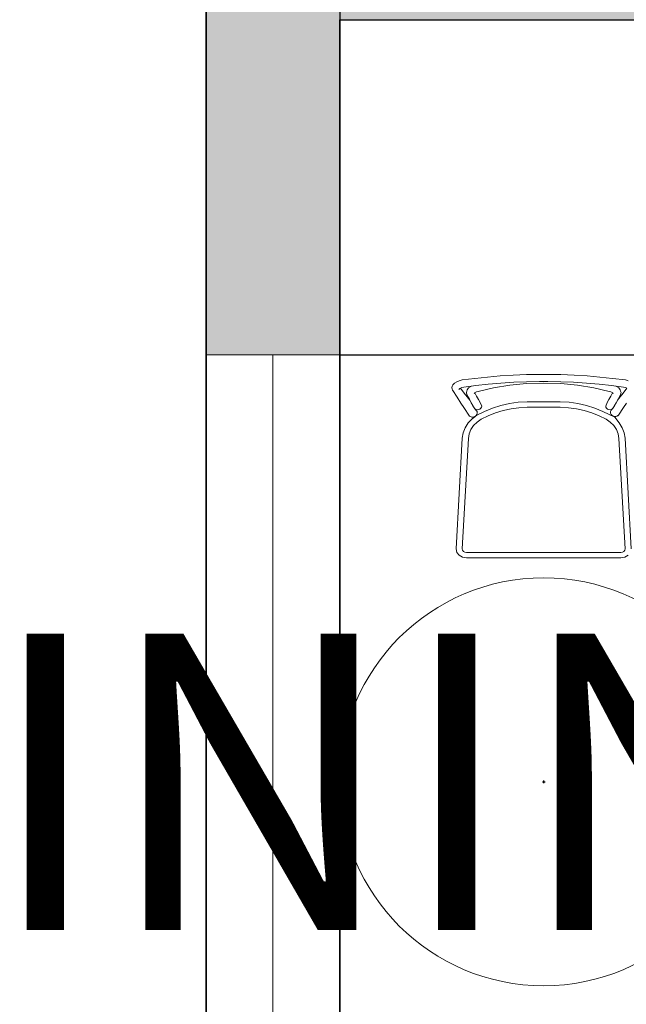
# Model space of a CAD drawing. Units: inches. Extents: x 305 to 776, y 38 to 479.
# Tile 7 of 14: x 378 to 419, y 265 to 332. Entities that reach past the tile are written whole.
import ezdxf

# ---------------------------------------------------------------- set-up
doc = ezdxf.new("R2010")
doc.units = ezdxf.units.IN
doc.header["$MEASUREMENT"] = 0
for name, color, linetype, lineweight in [('A-ANNO-DIMS', 2, 'Continuous', 18), ('A-FURN', 8, 'Continuous', 18), ('A-GLAZ', 4, 'Continuous', 20), ('A-WALL', 7, 'Continuous', 35), ('A-WALL-PATT', 252, 'Continuous', 13)]:
    doc.layers.add(name, color=color, linetype=linetype, lineweight=lineweight)
doc.styles.get("Standard").update_dxf_attribs({"font": 'arial.ttf'})
doc.dimstyles.get("Standard").update_dxf_attribs({"dimtxt": 20, "dimasz": 0.18, "dimexe": 0.18, "dimexo": 0.0625, "dimgap": 0.09, "dimtad": 0, "dimtih": 1, "dimtoh": 1, "dimdec": 4, "dimzin": 0, "dimdsep": 46, "dimtxsty": 'Standard', "dimcen": 0.09, "dimadec": 0, "dimazin": 0, "dimtfac": 1, "dimtdec": 4, "dimtofl": 0, "dimtmove": 0, "dimatfit": 3, "dimfxl": 1, "dimtolj": 1, "dimtzin": 0, "dimarcsym": 0})

# ---------------------------------------------------------------- blocks, each defined once
blk = doc.blocks.new('W3')
for p, q in [((867.012, 308.312), (847.412, 308.312)), ((886.612, 308.312), (867.012, 308.312)), ((906.212, 308.312), (886.612, 308.312))]:
    blk.add_line(p, q)
for points in [[(867.012, 312.812), (847.412, 312.812), (847.412, 303.812), (867.012, 303.812)], [(886.612, 312.812), (867.012, 312.812)], [(886.612, 303.812), (906.212, 303.812), (906.212, 312.812), (886.612, 312.812)], [(867.012, 303.812), (886.612, 303.812)]]:
    blk.add_lwpolyline(points)
blk = doc.blocks.new('D')
for p, q in [((1074.023, 532.53), (1074.289, 532.604)), ((1074.289, 532.603), (1074.023, 532.529)), ((1074.289, 532.604), (1075.47, 532.753)), ((1075.47, 532.752), (1074.289, 532.603)), ((1075.47, 532.753), (1076.649, 532.882)), ((1076.649, 532.881), (1075.47, 532.752)), ((1077.847, 532.985), (1076.649, 532.881)), ((1076.649, 532.882), (1077.847, 532.985)), ((1077.847, 532.985), (1079.059, 533.061)), ((1079.059, 533.06), (1077.847, 532.985)), ((1079.059, 533.061), (1080.28, 533.107)), ((1080.28, 533.106), (1079.059, 533.06)), ((1080.28, 533.107), (1081.503, 533.122)), ((1081.503, 533.121), (1080.28, 533.106)), ((1081.503, 533.122), (1082.266, 533.122)), ((1082.266, 533.121), (1081.503, 533.121)), ((1083.489, 533.107), (1082.266, 533.122)), ((1083.489, 533.106), (1082.266, 533.121)), ((1084.71, 533.061), (1083.489, 533.107)), ((1084.71, 533.06), (1083.489, 533.106)), ((1085.922, 532.985), (1084.71, 533.061)), ((1085.922, 532.985), (1084.71, 533.06)), ((1087.12, 532.881), (1085.922, 532.985)), ((1087.12, 532.882), (1085.922, 532.985)), ((1088.299, 532.753), (1087.12, 532.882)), ((1088.299, 532.752), (1087.12, 532.881)), ((1089.48, 532.604), (1088.299, 532.753)), ((1089.48, 532.603), (1088.299, 532.752)), ((1089.746, 532.53), (1089.48, 532.604)), ((1089.746, 532.529), (1089.48, 532.603)), ((1073.341, 531.888), (1073.376, 532.016)), ((1073.376, 532.015), (1073.341, 531.888)), ((1073.341, 531.888), (1073.369, 531.767)), ((1073.341, 531.888), (1073.369, 531.768)), ((1073.402, 531.662), (1073.369, 531.768)), ((1073.369, 531.767), (1073.402, 531.661)), ((1073.376, 532.016), (1073.421, 532.144)), ((1073.421, 532.143), (1073.376, 532.015)), ((1073.402, 531.662), (1073.441, 531.614)), ((1073.402, 531.661), (1073.441, 531.613)), ((1073.421, 532.144), (1073.589, 532.32)), ((1073.589, 532.319), (1073.421, 532.143)), ((1073.589, 532.32), (1073.794, 532.442)), ((1073.794, 532.441), (1073.589, 532.319)), ((1073.794, 532.442), (1074.023, 532.53)), ((1074.023, 532.529), (1073.794, 532.441)), ((1073.99, 531.719), (1074.082, 531.807)), ((1074.082, 531.807), (1074.149, 531.847)), ((1074.149, 531.847), (1074.284, 531.898)), ((1074.503, 531.382), (1074.155, 531.849)), ((1074.284, 531.898), (1074.454, 531.945)), ((1074.454, 531.945), (1075.569, 532.086)), ((1074.727, 531.568), (1074.764, 531.683)), ((1074.764, 531.683), (1074.907, 531.863)), ((1074.907, 531.863), (1075.103, 532.007)), ((1075.103, 532.007), (1075.165, 532.035)), ((1075.569, 532.086), (1076.732, 532.213)), ((1075.79, 531.547), (1077.219, 531.872)), ((1076.732, 532.213), (1077.91, 532.315)), ((1077.219, 531.872), (1078.734, 532.121)), ((1077.91, 532.315), (1079.101, 532.389)), ((1078.734, 532.121), (1080.296, 532.268)), ((1079.101, 532.389), (1080.302, 532.434)), ((1080.296, 532.268), (1081.884, 532.303)), ((1080.302, 532.434), (1081.509, 532.449)), ((1081.509, 532.449), (1082.26, 532.449)), ((1083.473, 532.268), (1081.884, 532.303)), ((1083.467, 532.434), (1082.26, 532.449)), ((1084.668, 532.389), (1083.467, 532.434)), ((1085.035, 532.121), (1083.473, 532.268)), ((1085.859, 532.315), (1084.668, 532.389)), ((1086.55, 531.872), (1085.035, 532.121)), ((1087.037, 532.213), (1085.859, 532.315)), ((1087.979, 531.547), (1086.55, 531.872)), ((1088.2, 532.086), (1087.037, 532.213)), ((1089.315, 531.945), (1088.2, 532.086)), ((1088.666, 532.007), (1088.604, 532.035)), ((1088.862, 531.863), (1088.666, 532.007)), ((1089.005, 531.683), (1088.862, 531.863)), ((1089.042, 531.568), (1089.005, 531.683)), ((1089.265, 531.382), (1089.614, 531.849)), ((1089.485, 531.898), (1089.315, 531.945)), ((1089.62, 531.847), (1089.485, 531.898)), ((1073.839, 531.004), (1073.441, 531.614)), ((1073.441, 531.613), (1073.839, 531.004)), ((1073.839, 531.004), (1074.192, 530.456)), ((1074.192, 530.457), (1073.839, 531.004)), ((1074.899, 530.868), (1074.503, 531.382)), ((1074.727, 531.568), (1074.693, 531.452)), ((1074.735, 531.227), (1074.693, 531.452)), ((1074.97, 530.808), (1074.735, 531.227)), ((1075.019, 530.719), (1074.899, 530.868)), ((1075.147, 530.489), (1074.97, 530.808)), ((1075.419, 531.311), (1075.441, 531.379)), ((1075.441, 531.379), (1075.456, 531.398)), ((1075.456, 531.398), (1075.511, 531.438)), ((1075.646, 531.109), (1075.472, 531.409)), ((1075.511, 531.438), (1075.628, 531.489)), ((1075.628, 531.489), (1075.79, 531.547)), ((1075.827, 530.783), (1075.646, 531.109)), ((1075.976, 530.506), (1075.827, 530.783)), ((1087.793, 530.506), (1087.942, 530.783)), ((1087.942, 530.783), (1088.123, 531.109)), ((1088.141, 531.489), (1087.979, 531.547)), ((1088.123, 531.109), (1088.297, 531.409)), ((1088.258, 531.438), (1088.141, 531.489)), ((1088.313, 531.398), (1088.258, 531.438)), ((1088.328, 531.379), (1088.313, 531.398)), ((1088.35, 531.311), (1088.328, 531.379)), ((1088.622, 530.489), (1088.799, 530.808)), ((1088.75, 530.719), (1088.87, 530.868)), ((1088.799, 530.808), (1089.034, 531.227)), ((1088.87, 530.868), (1089.265, 531.382)), ((1089.034, 531.227), (1089.076, 531.452)), ((1089.042, 531.568), (1089.076, 531.452)), ((1074.459, 530.031), (1074.192, 530.457)), ((1074.192, 530.456), (1074.459, 530.031)), ((1074.459, 530.031), (1074.997, 529.238)), ((1074.997, 529.239), (1074.459, 530.031)), ((1075.288, 530.225), (1075.147, 530.489)), ((1075.308, 530.194), (1075.288, 530.225)), ((1075.308, 530.194), (1075.415, 530.022)), ((1075.415, 530.022), (1075.489, 529.932)), ((1075.448, 529.974), (1075.614, 529.779)), ((1075.489, 529.932), (1075.593, 529.869)), ((1075.593, 529.869), (1075.714, 529.84)), ((1075.714, 529.84), (1075.839, 529.849)), ((1075.839, 529.849), (1075.954, 529.894)), ((1075.954, 529.894), (1076.045, 529.971)), ((1076.119, 530.181), (1075.976, 530.506)), ((1076.045, 529.971), (1076.102, 530.07)), ((1076.102, 530.07), (1076.119, 530.181)), ((1077.118, 529.996), (1076.372, 529.682)), ((1077.895, 530.244), (1077.118, 529.996)), ((1078.696, 530.423), (1077.895, 530.244)), ((1078.116, 529.763), (1078.845, 529.922)), ((1079.513, 530.531), (1078.696, 530.423)), ((1078.845, 529.922), (1079.588, 530.022)), ((1080.337, 530.567), (1079.513, 530.531)), ((1079.588, 530.022), (1080.337, 530.062)), ((1083.432, 530.567), (1080.337, 530.567)), ((1080.337, 530.062), (1083.432, 530.062)), ((1084.256, 530.531), (1083.432, 530.567)), ((1083.432, 530.062), (1084.181, 530.022)), ((1084.181, 530.022), (1084.924, 529.922)), ((1085.073, 530.423), (1084.256, 530.531)), ((1084.924, 529.922), (1085.653, 529.763)), ((1085.874, 530.244), (1085.073, 530.423)), ((1086.651, 529.996), (1085.874, 530.244)), ((1087.397, 529.682), (1086.651, 529.996)), ((1087.65, 530.181), (1087.793, 530.506)), ((1087.65, 530.181), (1087.667, 530.07)), ((1087.667, 530.07), (1087.724, 529.971)), ((1087.724, 529.971), (1087.815, 529.894)), ((1087.815, 529.894), (1087.93, 529.849)), ((1087.93, 529.849), (1088.055, 529.84)), ((1088.055, 529.84), (1088.176, 529.869)), ((1088.321, 529.974), (1088.159, 529.791)), ((1088.176, 529.869), (1088.28, 529.932)), ((1088.28, 529.932), (1088.354, 530.022)), ((1088.461, 530.194), (1088.354, 530.022)), ((1088.461, 530.194), (1088.481, 530.225)), ((1088.481, 530.225), (1088.622, 530.489)), ((1088.828, 529.323), (1089.31, 530.031)), ((1088.828, 529.323), (1089.31, 530.031)), ((1089.31, 530.031), (1089.577, 530.457)), ((1089.31, 530.031), (1089.577, 530.456)), ((1075.224, 528.986), (1074.859, 528.601)), ((1075.224, 528.985), (1074.859, 528.6)), ((1074.997, 529.239), (1075.136, 529.17)), ((1074.997, 529.238), (1075.064, 529.198)), ((1075.064, 529.198), (1075.138, 529.169)), ((1075.136, 529.17), (1075.294, 529.151)), ((1075.138, 529.169), (1075.217, 529.153)), ((1075.217, 529.153), (1075.297, 529.15)), ((1075.658, 529.323), (1075.224, 528.986)), ((1075.407, 529.127), (1075.224, 528.985)), ((1075.294, 529.151), (1075.448, 529.182)), ((1075.297, 529.15), (1075.377, 529.16)), ((1075.377, 529.16), (1075.407, 529.127)), ((1075.448, 529.182), (1075.58, 529.262)), ((1075.58, 529.262), (1075.671, 529.378)), ((1075.689, 529.655), (1075.614, 529.779)), ((1076.372, 529.682), (1075.658, 529.323)), ((1075.671, 529.378), (1075.709, 529.515)), ((1075.686, 528.68), (1076.065, 528.947)), ((1075.709, 529.515), (1075.689, 529.655)), ((1076.065, 528.947), (1076.72, 529.274)), ((1076.72, 529.274), (1077.406, 529.546)), ((1077.406, 529.546), (1078.116, 529.763)), ((1085.653, 529.763), (1086.363, 529.546)), ((1086.363, 529.546), (1087.049, 529.274)), ((1087.049, 529.274), (1087.704, 528.947)), ((1087.397, 529.682), (1088.507, 529.156)), ((1087.704, 528.947), (1088.083, 528.68)), ((1088.101, 529.662), (1088.098, 529.524)), ((1088.098, 529.524), (1088.153, 529.393)), ((1088.159, 529.791), (1088.101, 529.662)), ((1088.153, 529.393), (1088.256, 529.289)), ((1088.256, 529.289), (1088.394, 529.224)), ((1088.394, 529.224), (1088.549, 529.208)), ((1088.43, 529.192), (1088.443, 529.213)), ((1088.507, 529.156), (1088.43, 529.192)), ((1088.443, 529.213), (1088.513, 529.207)), ((1088.91, 528.6), (1088.507, 529.156)), ((1088.91, 528.601), (1088.507, 529.156)), ((1088.513, 529.207), (1088.583, 529.211)), ((1088.549, 529.208), (1088.701, 529.243)), ((1088.583, 529.211), (1088.651, 529.225)), ((1088.651, 529.225), (1088.716, 529.249)), ((1088.701, 529.243), (1088.828, 529.323)), ((1088.716, 529.249), (1088.775, 529.281)), ((1088.775, 529.281), (1088.828, 529.323)), ((1074.58, 528.163), (1074.397, 527.686)), ((1074.58, 528.162), (1074.397, 527.685)), ((1074.859, 528.601), (1074.58, 528.163)), ((1074.859, 528.6), (1074.58, 528.162)), ((1074.954, 527.587), (1075.116, 527.991)), ((1075.116, 527.991), (1075.363, 528.36)), ((1075.363, 528.36), (1075.686, 528.68)), ((1088.083, 528.68), (1088.406, 528.36)), ((1088.406, 528.36), (1088.653, 527.991)), ((1088.653, 527.991), (1088.815, 527.587)), ((1089.189, 528.163), (1088.91, 528.601)), ((1089.189, 528.162), (1088.91, 528.6)), ((1089.372, 527.686), (1089.189, 528.163)), ((1089.372, 527.685), (1089.189, 528.162)), ((1074.316, 527.187), (1073.749, 516.876)), ((1074.316, 527.186), (1073.749, 516.875)), ((1074.397, 527.686), (1074.316, 527.187)), ((1074.397, 527.685), (1074.316, 527.186)), ((1074.316, 516.876), (1074.883, 527.162)), ((1074.883, 527.162), (1074.954, 527.587)), ((1088.815, 527.587), (1088.886, 527.162)), ((1088.886, 527.162), (1089.453, 516.876)), ((1089.453, 527.187), (1089.372, 527.686)), ((1089.453, 527.186), (1089.372, 527.685)), ((1090.02, 516.876), (1089.453, 527.187)), ((1090.02, 516.875), (1089.453, 527.186)), ((1073.749, 516.876), (1073.821, 516.554)), ((1073.749, 516.875), (1073.821, 516.553)), ((1073.821, 516.554), (1074.026, 516.281)), ((1073.821, 516.553), (1074.026, 516.28)), ((1074.026, 516.281), (1074.333, 516.099)), ((1074.026, 516.28), (1074.333, 516.098)), ((1074.345, 516.747), (1074.316, 516.876)), ((1074.333, 516.099), (1074.695, 516.035)), ((1074.333, 516.098), (1074.695, 516.034)), ((1074.427, 516.638), (1074.345, 516.747)), ((1074.55, 516.565), (1074.427, 516.638)), ((1074.695, 516.539), (1074.55, 516.565)), ((1089.074, 516.539), (1074.695, 516.539)), ((1089.219, 516.565), (1089.074, 516.539)), ((1089.074, 516.035), (1089.436, 516.099)), ((1089.074, 516.034), (1089.436, 516.098)), ((1089.342, 516.638), (1089.219, 516.565)), ((1089.424, 516.747), (1089.342, 516.638)), ((1089.453, 516.876), (1089.424, 516.747)), ((1089.436, 516.099), (1089.743, 516.281)), ((1089.436, 516.098), (1089.743, 516.28)), ((1074.695, 516.035), (1089.074, 516.035)), ((1074.695, 516.034), (1089.074, 516.034))]:
    blk.add_line(p, q)
blk.add_circle((1081.884, 495.197), 18.987)
blk = doc.blocks.new('*D19')
at = {"layer": 'A-ANNO-DIMS', "color": 0, "lineweight": -2, "transparency": 16777216}
for p, q in [((557.633, 250.82), (557.633, 245.977)), ((589.133, 250.82), (589.133, 245.977)), ((557.633, 246.157), (557.453, 246.157)), ((588.953, 246.157), (557.813, 246.157))]:
    blk.add_line(p, q, dxfattribs=at)
at = {"layer": 'A-ANNO-DIMS', "color": 0, "transparency": 16777216}
for points in [[(557.813, 246.187), (557.813, 246.127), (557.633, 246.157)], [(588.953, 246.187), (588.953, 246.127), (589.133, 246.157)]]:
    blk.add_solid(points, dxfattribs=at)
at = {"layer": 'Defpoints', "color": 0, "transparency": 16777216}
for p in [(557.633, 250.882), (589.133, 250.882), (557.633, 246.157)]:
    blk.add_point(p, dxfattribs=at)
at = {"layer": 'A-ANNO-DIMS', "color": 0, "transparency": 16777216, "insert": (463.393, 246.157), "char_height": 20, "attachment_point": 5}
blk.add_mtext('\\A1;DOOR 32 TYP.', dxfattribs=at)
blk = doc.blocks.new('*D33')
at = {"layer": 'A-ANNO-DIMS', "color": 0, "lineweight": -2, "transparency": 16777216}
for p, q in [((440.927, 307.949), (449.29, 307.949)), ((449.11, 307.769), (449.11, 290.896)), ((449.11, 253.161), (449.11, 270.034)), ((440.927, 252.981), (449.29, 252.981))]:
    blk.add_line(p, q, dxfattribs=at)
at = {"layer": 'A-ANNO-DIMS', "color": 0, "transparency": 16777216}
for points in [[(449.08, 307.769), (449.14, 307.769), (449.11, 307.949)], [(449.08, 253.161), (449.14, 253.161), (449.11, 252.981)]]:
    blk.add_solid(points, dxfattribs=at)
at = {"layer": 'Defpoints', "color": 0, "transparency": 16777216}
for p in [(440.864, 307.949), (449.11, 307.949), (440.864, 252.981)]:
    blk.add_point(p, dxfattribs=at)
at = {"layer": 'A-ANNO-DIMS', "color": 0, "transparency": 16777216, "insert": (449.11, 280.465), "char_height": 20, "attachment_point": 5}
blk.add_mtext('\\A1;DINING SET 55', dxfattribs=at)
blk = doc.blocks.new('*D46')
at = {"layer": 'A-ANNO-DIMS', "color": 0, "lineweight": -2, "transparency": 16777216}
for p, q in [((390.57, 429.382), (372.451, 429.382)), ((372.631, 429.202), (372.631, 259.69)), ((372.631, 69.562), (372.631, 239.074)), ((390.57, 69.382), (372.451, 69.382))]:
    blk.add_line(p, q, dxfattribs=at)
at = {"layer": 'A-ANNO-DIMS', "color": 0, "transparency": 16777216}
for points in [[(372.601, 429.202), (372.661, 429.202), (372.631, 429.382)], [(372.601, 69.562), (372.661, 69.562), (372.631, 69.382)]]:
    blk.add_solid(points, dxfattribs=at)
at = {"layer": 'Defpoints', "color": 0, "transparency": 16777216}
for p in [(372.631, 429.382), (390.633, 429.382), (390.633, 69.382)]:
    blk.add_point(p, dxfattribs=at)
at = {"layer": 'A-ANNO-DIMS', "color": 0, "transparency": 16777216, "insert": (372.631, 249.382), "char_height": 20, "attachment_point": 5}
blk.add_mtext('\\A1;360', dxfattribs=at)
blk = doc.blocks.new('*D49')
at = {"layer": 'A-ANNO-DIMS', "color": 0, "lineweight": -2, "transparency": 16777216}
for p, q in [((399.695, 331.882), (648.814, 331.882)), ((648.634, 331.702), (648.634, 330.883)), ((648.634, 309.462), (648.634, 310.281)), ((399.695, 309.282), (648.814, 309.282))]:
    blk.add_line(p, q, dxfattribs=at)
at = {"layer": 'A-ANNO-DIMS', "color": 0, "transparency": 16777216}
for points in [[(648.604, 331.702), (648.664, 331.702), (648.634, 331.882)], [(648.604, 309.462), (648.664, 309.462), (648.634, 309.282)]]:
    blk.add_solid(points, dxfattribs=at)
at = {"layer": 'Defpoints', "color": 0, "transparency": 16777216}
for p in [(399.633, 331.882), (648.634, 331.882), (399.633, 309.282)]:
    blk.add_point(p, dxfattribs=at)
at = {"layer": 'A-ANNO-DIMS', "color": 0, "transparency": 16777216, "insert": (648.634, 320.582), "char_height": 20, "attachment_point": 5}
blk.add_mtext('\\A1;22.6', dxfattribs=at)
blk = doc.blocks.new('*D62')
at = {"layer": 'A-ANNO-DIMS', "color": 0, "lineweight": -2, "transparency": 16777216}
for p, q in [((399.633, 336.32), (399.633, 51.201)), ((423.233, 336.32), (423.233, 51.201)), ((399.813, 51.381), (423.053, 51.381)), ((423.233, 51.381), (423.413, 51.381))]:
    blk.add_line(p, q, dxfattribs=at)
at = {"layer": 'A-ANNO-DIMS', "color": 0, "transparency": 16777216}
for points in [[(399.813, 51.411), (399.813, 51.351), (399.633, 51.381)], [(423.053, 51.411), (423.053, 51.351), (423.233, 51.381)]]:
    blk.add_solid(points, dxfattribs=at)
at = {"layer": 'Defpoints', "color": 0, "transparency": 16777216}
for p in [(399.633, 336.382), (423.233, 336.382), (423.233, 51.381)]:
    blk.add_point(p, dxfattribs=at)
at = {"layer": 'A-ANNO-DIMS', "color": 0, "transparency": 16777216, "insert": (449.642, 51.381), "char_height": 20, "attachment_point": 5}
blk.add_mtext('\\A1;23.6', dxfattribs=at)
blk = doc.blocks.new('*D65')
at = {"layer": 'A-ANNO-DIMS', "color": 0, "lineweight": -2, "transparency": 16777216}
for p, q in [((399.633, 351.219), (399.633, 51.201)), ((421.89, 351.219), (421.89, 51.201)), ((399.813, 51.381), (421.71, 51.381)), ((421.89, 51.381), (422.07, 51.381))]:
    blk.add_line(p, q, dxfattribs=at)
at = {"layer": 'A-ANNO-DIMS', "color": 0, "transparency": 16777216}
for points in [[(399.813, 51.411), (399.813, 51.351), (399.633, 51.381)], [(421.71, 51.411), (421.71, 51.351), (421.89, 51.381)]]:
    blk.add_solid(points, dxfattribs=at)
at = {"layer": 'Defpoints', "color": 0, "transparency": 16777216}
for p in [(399.633, 351.281), (421.89, 351.281), (421.89, 51.381)]:
    blk.add_point(p, dxfattribs=at)
at = {"layer": 'A-ANNO-DIMS', "color": 0, "transparency": 16777216, "insert": (463.844, 51.381), "char_height": 20, "attachment_point": 5}
blk.add_mtext('\\A1;22.257', dxfattribs=at)
blk = doc.blocks.new('*D75')
at = {"layer": 'A-ANNO-DIMS', "color": 0, "lineweight": -2, "transparency": 16777216}
for p, q in [((413.291, 280.465), (413.471, 280.465)), ((413.381, 280.375), (413.381, 280.555)), ((435.396, 280.465), (427.32, 280.465))]:
    blk.add_line(p, q, dxfattribs=at)
at = {"layer": 'A-ANNO-DIMS', "color": 0, "transparency": 16777216}
blk.add_solid([(427.32, 280.495), (427.32, 280.435), (427.14, 280.465)], dxfattribs=at)
at = {"layer": 'Defpoints', "color": 0, "transparency": 16777216}
for p in [(399.621, 280.466), (427.14, 280.465)]:
    blk.add_point(p, dxfattribs=at)
at = {"layer": 'A-ANNO-DIMS', "color": 0, "transparency": 16777216, "insert": (480.009, 280.465), "char_height": 20, "attachment_point": 5}
blk.add_mtext('\\A1;∅27.52', dxfattribs=at)

msp = doc.modelspace()

# ---------------------------------------------------------------- hatches: boundary and pattern name
at = {"layer": 'A-WALL-PATT'}
h = msp.add_hatch(color=256, dxfattribs=at)
h.dxf.hatch_style = 1
h.paths.add_polyline_path([(481.3329, 429.382), (390.6329, 429.382), (390.6329, 398.067), (399.6329, 398.067), (399.6329, 420.382), (465.6329, 420.382), (465.6329, 331.882), (470.1329, 331.882), (470.1329, 355.882), (512.1329, 355.882), (512.1329, 337.282), (512.1329, 337.282), (515.8592, 337.282), (516.6329, 337.282), (516.6329, 360.382), (513.3171, 360.382), (470.1329, 360.382), (470.1329, 420.382), (481.3329, 420.382)])
h.paths.add_polyline_path([(630.6329, 429.382), (500.9329, 429.382), (500.9329, 420.382), (502.8693, 420.382), (512.1329, 420.382), (512.1329, 391.882), (516.6329, 391.882), (516.6329, 420.382), (621.6329, 420.382), (621.6329, 388.182), (630.6329, 388.182)])
h.paths.add_polyline_path([(630.6329, 329.382), (621.6329, 329.382), (621.6329, 301.882), (512.1329, 301.882), (512.1329, 297.382), (515.8592, 297.382), (557.6329, 297.382), (621.6329, 297.382), (621.6329, 286.182), (630.6329, 286.182)])
h.paths.add_polyline_path([(630.6329, 266.582), (621.6329, 266.582), (621.6329, 255.382), (589.1329, 255.382), (589.1329, 250.882), (621.6329, 250.882), (621.6329, 226.282), (630.6329, 226.282)])
h.paths.add_polyline_path([(630.6329, 167.482), (621.6329, 167.482), (621.6329, 149.1444), (621.6329, 142.882), (516.6329, 142.882), (516.6329, 261.982), (512.1329, 261.982), (512.1329, 138.382), (621.6329, 138.382), (621.6329, 78.382), (512.1329, 78.382), (512.1329, 69.382), (630.6329, 69.382)])
h.paths.add_polyline_path([(464.1329, 138.382), (476.7329, 138.382), (476.7329, 142.1084), (476.7329, 142.882), (459.6329, 142.882), (459.6329, 78.382), (399.6329, 78.382), (399.6329, 98.582), (390.6329, 98.582), (390.6329, 69.382), (464.1329, 69.382)])
h.paths.add_polyline_path([(459.6329, 142.882), (439.3329, 142.882), (439.3329, 138.382), (459.6329, 138.382)], flags=17)
h.paths.add_polyline_path([(399.6329, 138.382), (403.9329, 138.382), (403.9329, 141.5545), (403.9329, 141.5545), (403.9329, 142.882), (399.6329, 142.882), (399.6329, 250.4819), (390.6329, 250.4819), (390.6329, 118.182), (399.6329, 118.182)])
h.paths.add_polyline_path([(399.6329, 331.882), (428.2629, 331.882), (428.2629, 336.382), (399.6329, 336.382), (399.6329, 358.697), (390.6329, 358.697), (390.6329, 309.2819), (399.6329, 309.2819)])

# ---------------------------------------------------------------- linework, layer by layer
at = {"layer": 'A-WALL'}
msp.add_line((399.6329, 331.882), (399.6329, 142.882), dxfattribs=at)
msp.add_lwpolyline([(390.6329, 69.382), (630.6329, 69.382), (630.6329, 429.382), (390.6329, 429.382)], close=True, dxfattribs=at)

# ---------------------------------------------------------------- block references
at = {"layer": 'A-FURN', "xscale": 0.724692399516523, "yscale": 0.724692399516523, "zscale": 0.724692399516523}
msp.add_blockref('D', (-370.653, -78.4001), dxfattribs=at)
at = {"layer": 'A-GLAZ', "rotation": 270}
msp.add_blockref('W3', (86.8213, 1156.694), dxfattribs=at)

# ---------------------------------------------------------------- dimensions: what is measured, and where the dimension line sits
at = {"layer": 'A-ANNO-DIMS'}
for base, p1, p2, override, picture, middle in [((372.6314, 429.382), (390.6329, 69.382), (390.6329, 429.382), {"dimdec": 0, "dimlfac": 1, "dimrnd": 0, "dimzin": 0, "dimdsep": 46, "dimlunit": 2}, '*D46', (372.6314, 249.382)), ((648.6344, 331.882), (399.6329, 309.2819), (399.6329, 331.882), {"dimdec": 1, "dimlfac": 1, "dimrnd": 0, "dimzin": 0, "dimdsep": 46, "dimlunit": 2}, '*D49', (648.6344, 320.582))]:
    dim = msp.add_linear_dim(base=base, p1=p1, p2=p2, angle=90, dimstyle='Standard', override=override, dxfattribs=at)
    dim.commit()
    dim.dimension.update_dxf_attribs({"geometry": picture, "text_midpoint": middle})
for base, p1, p2, override, picture, middle in [((421.8895, 51.3805), (399.6329, 351.2815), (421.8895, 351.2815), {"dimdec": 3, "dimlfac": 1, "dimrnd": 0, "dimzin": 0, "dimdsep": 46, "dimlunit": 2}, '*D65', (463.8444, 51.3805)), ((423.2329, 51.3805), (399.6329, 336.382), (423.2329, 336.382), {"dimdec": 1, "dimlfac": 1, "dimrnd": 0, "dimzin": 0, "dimdsep": 46, "dimlunit": 2}, '*D62', (449.6421, 51.3805))]:
    dim = msp.add_linear_dim(base=base, p1=p1, p2=p2, dimstyle='Standard', override=override, dxfattribs=at)
    dim.commit()
    dim.dimension.update_dxf_attribs({"geometry": picture, "text_midpoint": middle})
for base, p1, p2, angle, text, picture, middle in [((449.1096, 307.9493), (440.8644, 252.9815), (440.8644, 307.9493), 90, 'DINING SET <>', '*D33', (449.1096, 280.4654)), ((557.6329062952, 246.15704135), (589.1329062952, 250.88204135), (557.6329062952, 250.88204135), 180, 'DOOR <> TYP.', '*D19', (463.3929199378, 246.15704135))]:
    dim = msp.add_linear_dim(base=base, p1=p1, p2=p2, angle=angle, text=text, dimstyle='Standard', override={"dimdec": 0, "dimlfac": 1, "dimrnd": 0, "dimzin": 0, "dimdsep": 46, "dimlunit": 2}, dxfattribs=at)
    dim.commit()
    dim.dimension.update_dxf_attribs({"geometry": picture, "text_midpoint": middle})
dim = msp.add_diameter_dim_2p(p1=(399.6205, 280.4658), p2=(427.1405, 280.465), dimstyle='Standard', override={"dimdec": 2, "dimlfac": 1, "dimrnd": 0, "dimzin": 0, "dimdsep": 46, "dimlunit": 2}, dxfattribs=at)
dim.commit()
dim.dimension.update_dxf_attribs({"geometry": '*D75', "text_midpoint": (435.3965, 280.4648), "dimtype": 163})

doc.saveas('drawing.dxf')
